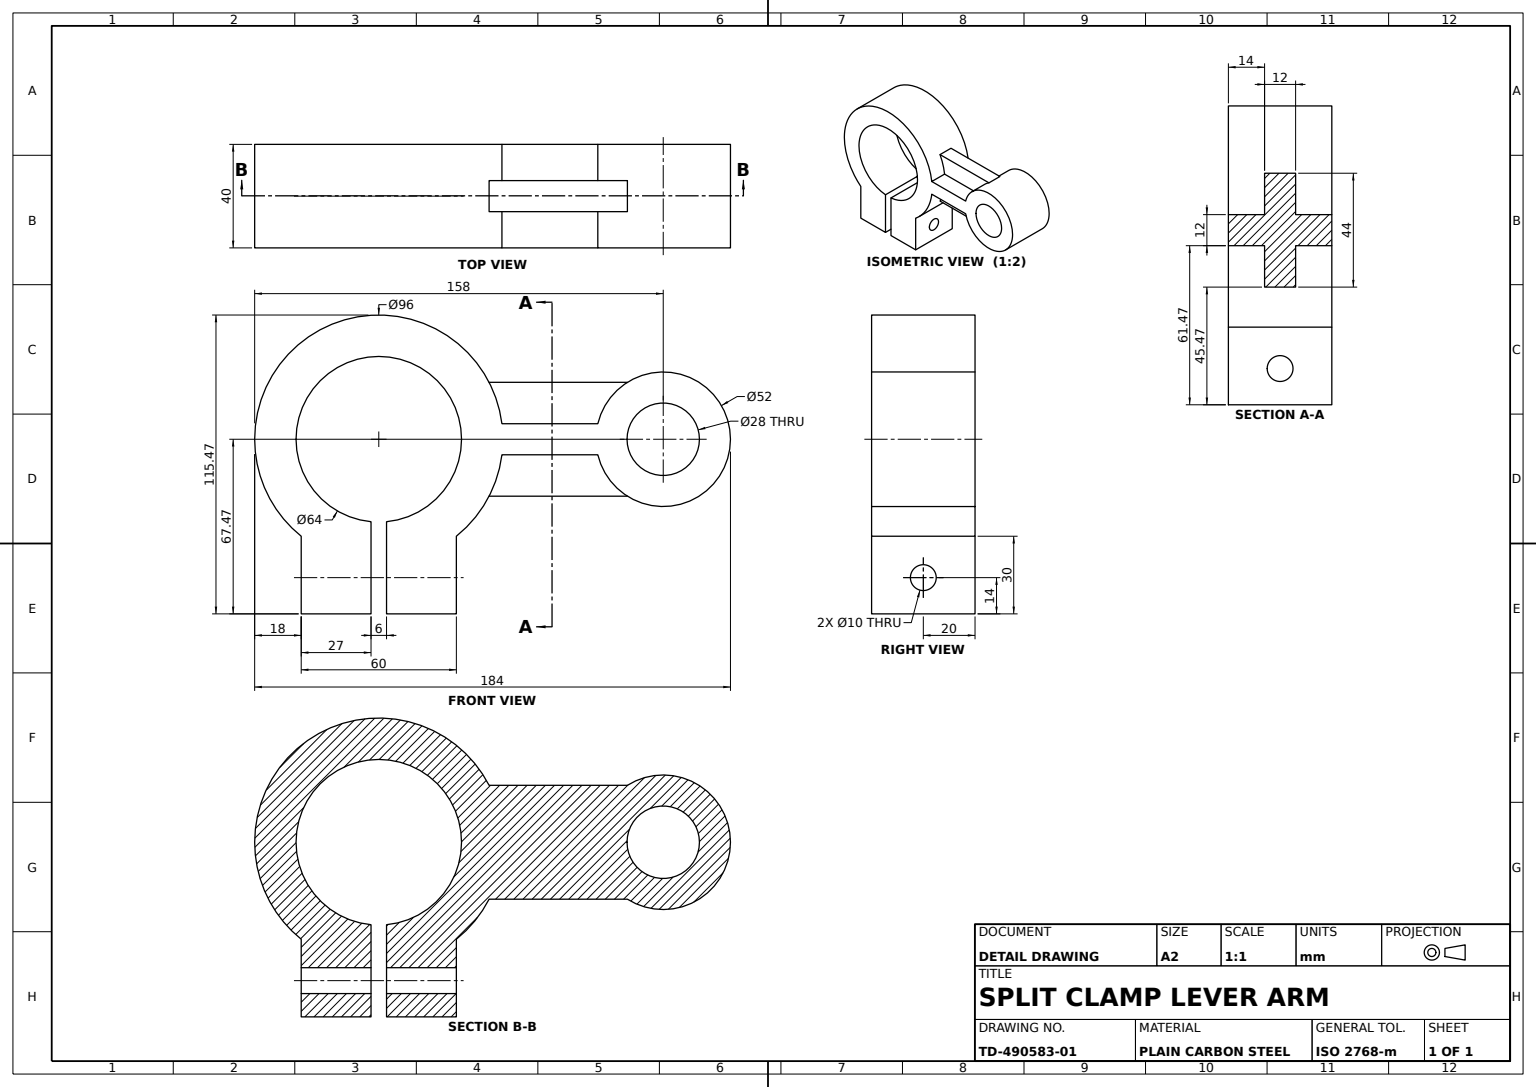
SolidWorks part; units mm, degrees
material "Plain Carbon Steel"
ref_plane "Front Plane" through (0, 0, 0) normal (0, 0, 1) x (1, 0, 0)
ref_plane "Top Plane" through (0, 0, 0) normal (0, 1, 0) x (1, 0, 0)
ref_plane "Right Plane" through (0, 0, 0) normal (1, 0, 0) x (0, 0, -1)
sketch "Clamp Ring Sketch" plane through (0, 0, 0) normal (0, 0, 1) x (1, 0, 0)
  circle A0 centre (0, 0) radius 48
  dimension "D1" = 96
  dimension "D2" = 96
extrude "Clamp Ring Ø96" add sketch "Clamp Ring Sketch" along normal blind 40
sketch "Clamp Lug Sketch" plane through (0, 0, 40) normal (0, 0, 1) x (1, 0, 0)
  line L0 (30, -67.47) -> (30, -37.47)
  line L1 (-30, -67.47) -> (-30, -37.47)
  line L3 (-30, -67.47) -> (30, -67.47)
  arc A1 (-30, -37.47) -> (30, -37.47) centre (0, 0) ccw
  dimension "D1" = 96
  dimension "D4" = 48
  dimension "D2" = 30
  dimension "D3" = 60
extrude "Clamp Lug" add sketch "Clamp Lug Sketch" against normal blind 40
sketch "Clamp Bore and Split Sketch" plane through (0, 0, 40) normal (0, 0, 1) x (1, 0, 0)
  line L0 (-3, -67.47) -> (3, -67.47)
  line L1 (-30, -67.47) -> (30, -67.47) construction
  line L2 (-30, -37.47) -> (-30, -67.47) construction
  line L3 (3, -67.47) -> (3, -31.8591)
  line L5 (-3, -31.8591) -> (-3, -67.47)
  arc A0 (3, -31.8591) -> (-3, -31.8591) centre (0, 0) ccw
  dimension "D1" = 64
  dimension "D2" = 32
  dimension "D3" = 27
extrude "Clamp Bore and Split Slot" cut sketch "Clamp Bore and Split Sketch" against normal blind 40
sketch "Pivot Eye Sketch" plane through (0, 0, 40) normal (0, 0, 1) x (1, 0, 0)
  line L0 (0, 0) -> (84, 0)
  line L1 (30, -67.47) -> (30, -37.47) construction
  circle A0 centre (110, 0) radius 26
  dimension "D1" = 52
  dimension "D2" = 52
  dimension "D3" = 54
extrude "Pivot Eye Ø52" add sketch "Pivot Eye Sketch" against normal blind 40 separate body contours A0
sketch "Connecting Arm Sketch" plane through (0, 0, 40) normal (0, 0, 1) x (1, 0, 0)
  line L0 (47.6235, 6) -> (84.7018, 6)
  line L5 (47.6235, -6) -> (84.7018, -6)
  circle A0 centre (110, 0) radius 26 construction
  arc A1 (84.7018, 6) -> (84.7018, -6) centre (110, 0) ccw
  arc A2 (47.6235, -6) -> (47.6235, 6) centre (0, 0) ccw
  dimension "D1" = 52
  dimension "D2" = 96
  dimension "D3" = 26
  dimension "D4" = 48
  dimension "D5" = 25.2982
extrude "Connecting Arm" add sketch "Connecting Arm Sketch" against normal blind 40
sketch "Arm Rib A Sketch" plane through (0, 6, 0) normal (0, 1, 0) x (1, 0, 0)
  line L0 (98.5168, -14) -> (110.3509, -14)
  line L1 (84.7018, 0) -> (84.7018, -40) construction
  line L2 (39.2684, -20) -> (39.2684, -14)
  line L3 (39.2684, -14) -> (98.5168, -14)
  line L5 (98.5168, -26) -> (39.2684, -26)
  line L6 (39.2684, -26) -> (39.2684, -20)
  line L7 (110.3509, -14) -> (110.3509, -26)
  line L8 (110.3509, -26) -> (98.5168, -26)
  line L9 (84.7018, -40) -> (47.6235, -40) construction
  dimension "D1" = 13.815
  dimension "D2" = 25.6491
  dimension "D3" = 45.4334
  dimension "D4" = 14
  dimension "D5" = 20
extrude "Arm Rib A" add sketch "Arm Rib A Sketch" along normal blind 16
sketch "Arm Rib B Sketch" plane through (0, -6, 0) normal (0, -1, 0) x (1, 0, 0)
  line L0 (47.6235, 0) -> (47.6235, 40) construction
  line L1 (47.6235, 40) -> (84.7018, 40) construction
  line L2 (38.2397, 20) -> (38.2397, 26)
  line L3 (38.2397, 26) -> (110.3509, 26)
  line L4 (110.3509, 26) -> (110.3509, 14)
  line L5 (110.3509, 14) -> (38.2397, 14)
  line L6 (38.2397, 14) -> (38.2397, 20)
  dimension "D1" = 62.7274
  dimension "D2" = 9.3838
  dimension "D3" = 14
  dimension "D4" = 20
extrude "Arm Rib B" add sketch "Arm Rib B Sketch" along normal blind 16
sketch "Pivot Bore Sketch" plane through (0, 0, 40) normal (0, 0, 1) x (1, 0, 0)
  circle A0 centre (110, 0) radius 14
  dimension "D1" = 28
  dimension "D2" = 28
extrude "Pivot Bore Ø28" cut sketch "Pivot Bore Sketch" against normal blind 40
sketch "Clamp Screw Hole Sketch" plane through (30, 0, 0) normal (1, 0, 0) x (0, 0, -1)
  line L0 (0, -67.47) -> (-40, -67.47) construction
  line L1 (-40, -67.47) -> (-40, -37.47) construction
  circle A0 centre (-20, -53.47) radius 5
  dimension "D1" = 10
  dimension "D2" = 14
  dimension "D4" = 10
  dimension "D3" = 20
extrude "Clamp Screw Hole Ø10" cut sketch "Clamp Screw Hole Sketch" against normal blind 80
